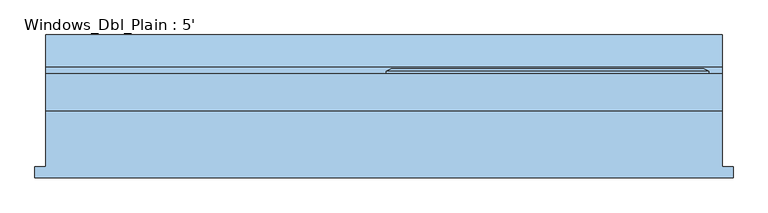
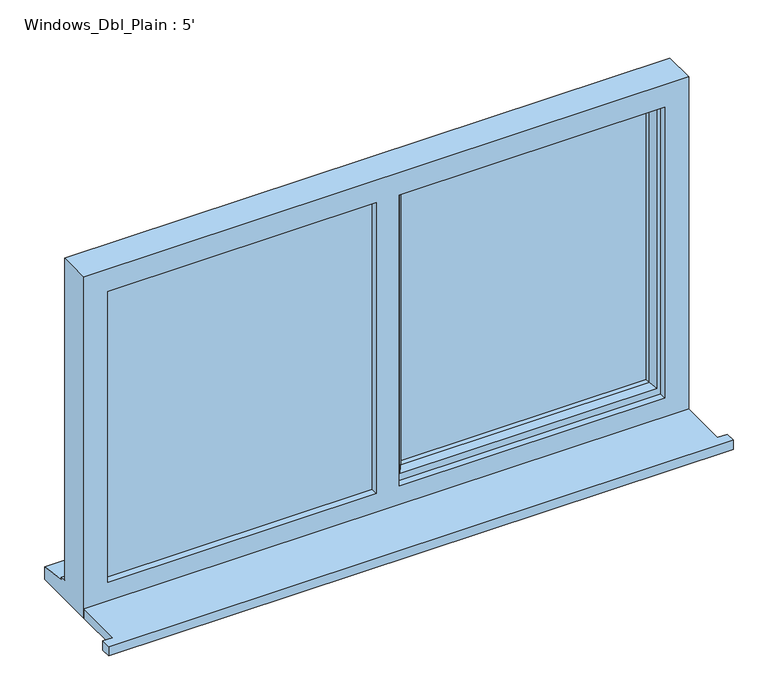
"""IFC4 building model written with IfcOpenShell, lengths in millimetres: window geometry, Windows_Dbl_Plain : 5'."""

from ifc_helpers import new_model, si_unit, frame, origin, place, context, project, spatial, polyline, outline, extrude, faceted_brep, source, transform, mapped, element, save


def windows_dbl_plain_5_b9c38b89(model_context):
    return source(origin(), model_context, "Body", "SolidModel", [
        extrude(outline(polyline([(-1072.0, -146.0834322), (-1072.0, -121.0834322), (-1047.0, -121.0834322), (-1047.0, 4.9965678), (477.0, 4.9965678), (477.0, -121.0834322), (502.0, -121.0834322), (502.0, -146.0834322), (-1072.0, -146.0834322)])), frame((0.0, 0.0, 1200.0), z_axis=(0.0, 0.0, 1.0), x_axis=(1.0, 0.0, 0.0)), (0.0, 0.0, 1.0), 25.0),
        faceted_brep([(-280.0, 87.9965678, 2080.0), (-280.0, 93.7700705, 2080.0), (-280.0, 93.7700705, 1253.0), (-280.0, 87.9965678, 1253.0), (-270.0, 22.9965678, 2070.0), (-270.0, 87.9965678, 2070.0), (-270.0, 87.9965678, 1263.0), (-270.0, 22.9965678, 1263.0), (-230.0, 37.4894677, 2030.0), (-240.1480377, 22.9965678, 2040.1480377), (-240.1480377, 22.9965678, 1292.8519623), (-230.0, 37.4894677, 1303.0), (-230.0, 51.9965678, 2030.0), (-230.0, 51.9965678, 1303.0), (-240.0, 75.9965678, 2040.0), (-240.0, 51.9965678, 2040.0), (-240.0, 51.9965678, 1293.0), (-240.0, 75.9965678, 1293.0), (-230.0, 93.7700705, 2030.0), (-230.0, 75.9965678, 2030.0), (-230.0, 75.9965678, 1303.0), (-230.0, 93.7700705, 1303.0), (-247.4457548, 99.5435732, 2047.4457548), (-247.4457548, 99.5435732, 1285.5542452), (-269.2153903, 99.5435732, 2069.2153903), (-269.2153903, 99.5435732, 1263.7846097), (447.0, 93.7700705, 1253.0), (447.0, 87.9965678, 1253.0), (437.0, 87.9965678, 1263.0), (437.0, 22.9965678, 1263.0), (407.1480377, 22.9965678, 1292.8519623), (397.0, 37.4894677, 1303.0), (397.0, 51.9965678, 1303.0), (407.0, 51.9965678, 1293.0), (407.0, 75.9965678, 1293.0), (397.0, 75.9965678, 1303.0), (397.0, 93.7700705, 1303.0), (414.4457548, 99.5435732, 1285.5542452), (436.2153903, 99.5435732, 1263.7846097), (447.0, 93.7700705, 2080.0), (447.0, 87.9965678, 2080.0), (437.0, 87.9965678, 2070.0), (437.0, 22.9965678, 2070.0), (407.1480377, 22.9965678, 2040.1480377), (397.0, 37.4894677, 2030.0), (397.0, 51.9965678, 2030.0), (407.0, 51.9965678, 2040.0), (407.0, 75.9965678, 2040.0), (397.0, 75.9965678, 2030.0), (397.0, 93.7700705, 2030.0), (414.4457548, 99.5435732, 2047.4457548), (436.2153903, 99.5435732, 2069.2153903)], [[[0, 1, 2, 3]], [[4, 5, 6, 7]], [[8, 9, 10, 11]], [[12, 8, 11, 13]], [[14, 15, 16, 17]], [[18, 19, 20, 21]], [[22, 18, 21, 23]], [[1, 24, 25, 2]], [[3, 2, 26, 27]], [[7, 6, 28, 29]], [[11, 10, 30, 31]], [[13, 11, 31, 32]], [[17, 16, 33, 34]], [[21, 20, 35, 36]], [[23, 21, 36, 37]], [[2, 25, 38, 26]], [[27, 26, 39, 40]], [[29, 28, 41, 42]], [[31, 30, 43, 44]], [[32, 31, 44, 45]], [[34, 33, 46, 47]], [[36, 35, 48, 49]], [[37, 36, 49, 50]], [[26, 38, 51, 39]], [[40, 39, 1, 0]], [[3, 27, 40, 0], [5, 41, 28, 6]], [[42, 41, 5, 4]], [[7, 29, 42, 4], [9, 43, 30, 10]], [[44, 43, 9, 8]], [[45, 44, 8, 12]], [[15, 46, 33, 16], [13, 32, 45, 12]], [[47, 46, 15, 14]], [[17, 34, 47, 14], [19, 48, 35, 20]], [[49, 48, 19, 18]], [[50, 49, 18, 22]], [[24, 51, 38, 25], [23, 37, 50, 22]], [[39, 51, 24, 1]]]),
        extrude(outline(polyline([(2050.0, -310.0), (2070.0, -310.0), (2070.0, -1007.0), (1263.0, -1007.0), (1263.0, -310.0), (1283.0, -310.0), (1283.0, -987.0), (2050.0, -987.0), (2050.0, -310.0)])), frame((0.0, 46.9965678, 0.0), z_axis=(0.0, 1.0, 0.0), x_axis=(0.0, 0.0, 1.0)), (0.0, 0.0, 1.0), 41.0),
        faceted_brep([(477.0, 4.9965678, 2110.0), (-1047.0, 4.9965678, 2110.0), (-1047.0, 4.9965678, 1200.0), (477.0, 4.9965678, 1200.0), (417.0, 4.9965678, 2050.0), (417.0, 4.9965678, 1275.0), (-252.0, 4.9965678, 1275.0), (-252.0, 4.9965678, 2050.0), (-310.0, 4.9965678, 2050.0), (-310.0, 4.9965678, 1275.0), (-987.0, 4.9965678, 1275.0), (-987.0, 4.9965678, 2050.0), (-1047.0, 87.9965678, 2110.0), (-1047.0, 87.9965678, 1251.0), (-1047.0, 102.9965678, 1249.68767), (-1047.0, 102.9965678, 1244.7449676), (-1047.0, 175.4965678, 1233.8088847), (-1047.0, 175.4965678, 1200.0), (477.0, 87.9965678, 2110.0), (477.0, 87.9965678, 1251.0), (-1007.0, 87.9965678, 2070.0), (-1007.0, 87.9965678, 1263.0), (-310.0, 87.9965678, 1263.0), (-310.0, 87.9965678, 2070.0), (-270.0, 87.9965678, 2070.0), (-270.0, 87.9965678, 1263.0), (437.0, 87.9965678, 1263.0), (437.0, 87.9965678, 2070.0), (-1007.0, 22.9965678, 2070.0), (-1007.0, 22.9965678, 1263.0), (-300.0, 22.9965678, 2070.0), (-300.0, 22.9965678, 1263.0), (-310.0, 22.9965678, 2050.0), (-987.0, 22.9965678, 2050.0), (-987.0, 22.9965678, 1275.0), (-310.0, 22.9965678, 1275.0), (-270.0, 22.9965678, 2070.0), (437.0, 22.9965678, 2070.0), (437.0, 22.9965678, 1263.0), (-270.0, 22.9965678, 1263.0), (417.0, 22.9965678, 2050.0), (-252.0, 22.9965678, 2050.0), (-252.0, 22.9965678, 1275.0), (417.0, 22.9965678, 1275.0), (-310.0, 46.9965678, 2070.0), (-300.0, 46.9965678, 2070.0), (477.0, 175.4965678, 1200.0), (477.0, 175.4965678, 1233.8088847), (477.0, 102.9965678, 1244.7449676), (477.0, 102.9965678, 1249.68767), (-300.0, 46.9965678, 1263.0), (-310.0, 46.9965678, 1263.0)], [[[0, 1, 2, 3], [4, 5, 6, 7], [8, 9, 10, 11]], [[2, 1, 12, 13, 14, 15, 16, 17]], [[13, 12, 18, 19], [20, 21, 22, 23], [24, 25, 26, 27]], [[21, 20, 28, 29]], [[28, 30, 31, 29], [32, 33, 34, 35]], [[36, 37, 38, 39], [40, 41, 42, 43]], [[33, 11, 10, 34]], [[1, 0, 18, 12]], [[28, 20, 23, 44, 45, 30]], [[27, 37, 36, 24]], [[11, 33, 32, 8]], [[40, 4, 7, 41]], [[19, 18, 0, 3, 46, 47, 48, 49]], [[27, 26, 38, 37]], [[4, 40, 43, 5]], [[45, 50, 31, 30]], [[50, 45, 44, 51]], [[51, 44, 23, 22]], [[25, 24, 36, 39]], [[41, 7, 6, 42]], [[8, 32, 35, 9]], [[46, 3, 2, 17]], [[47, 46, 17, 16]], [[48, 47, 16, 15]], [[49, 48, 15, 14]], [[19, 49, 14, 13]], [[22, 21, 29, 31, 50, 51]], [[26, 25, 39, 38]], [[6, 5, 43, 42]], [[35, 34, 10, 9]]]),
        extrude(outline(polyline([(-1007.0, 46.9965678), (-300.0, 46.9965678), (-300.0, 22.9965678), (-1007.0, 22.9965678), (-1007.0, 46.9965678)])), frame((0.0, 0.0, 1263.0), z_axis=(0.0, 0.0, 1.0), x_axis=(1.0, 0.0, 0.0)), (0.0, 0.0, 1.0), 807.0),
        extrude(outline(polyline([(407.0, 51.9965678), (-240.0, 51.9965678), (-240.0, 75.9965678), (407.0, 75.9965678), (407.0, 51.9965678)])), frame((0.0, 0.0, 1293.0), z_axis=(0.0, 0.0, 1.0), x_axis=(1.0, 0.0, 0.0)), (0.0, 0.0, 1.0), 747.0),
    ])


if __name__ == "__main__":
    model = new_model("IFC4")
    model_context = context("Model", 3, world=origin())
    ifc_project = project(units=[si_unit("LENGTHUNIT", "METRE", prefix="MILLI")], contexts=[model_context])
    site = spatial("IfcSite", under=ifc_project)
    building = spatial("IfcBuilding", under=site)
    placement = place(None, origin())
    windows_dbl_plain_5_shape = windows_dbl_plain_5_b9c38b89(model_context)
    element("IfcWindow", 1, ObjectType="Windows_Dbl_Plain : 5'", at=placement, inside=building, context=model_context, shape_type="MappedRepresentation", body=[
        mapped(windows_dbl_plain_5_shape, transform((0.0, 0.0, 0.0), x_axis=(1.0, 0.0, 0.0), y_axis=(0.0, 1.0, 0.0), z_axis=(0.0, 0.0, 1.0))),
    ])
    save(model, "model.ifc")

# Revit data of these elements
# Type "Windows_Dbl_Plain : 5'"
#   Type Mark = "62"
#   Operation = "DoublePanelVertical"
#   Construction Type Id = "GSP4R"
#   Manufacturer = "Revit"
#   Keynote = "L10"
#   Analytic Construction = "1/8 in Pilkington single glazing"
#   Wrap Layers (Ext) from Ext = 102.5 mm
#   Wrap Layers (Int) from Ext = 177.5 mm
#   Window Board Projection = 25 mm
#   Window Board Extension = 25 mm
#   Visual Light Transmittance = 0.9
#   Solar Heat Gain Coefficient = 0.78
#   Rough Width = 1524 mm
#   Rough Height = 910 mm
#   Height = 910 mm
#   Width = 1524 mm
#   Heat Transfer Coefficient (U) = 3.6886 W/(m²·K)
#   Glazing Thickness = 24 mm
#   FrameOffset - External = 50 mm
#   Frame Depth = 65 mm
#   Default Head Height = 2110 mm
#   Cill Depth = 87.5 mm
#   Cavity Closer Width = 50 mm
#   Cavity Closer Offset from Ext = 102.5 mm
#   Cavity Closer Depth = 85 mm
#   Vis - Cavity Closers = yes
#   Define Thermal Properties by = 1
#   Material Trim = Window Frame
#   Material Glass = Glass
#   Material Frame = Window Frame
#   Wall Closure = (empty or 0)
# Element 1 (IfcWindow, "Windows_Dbl_Plain : 5'")
#   Materials on its faces: "Window Frame", "Glass"
# Materials
#   "Window Frame": colour RGB 249 249 249, transparency 0, Keynote = "L10", Cost = 0
#   "Glass": class "Glass", colour RGB 0 128 192, transparency 0.9, Description = "Soda Lime Glass", Cost = 0
